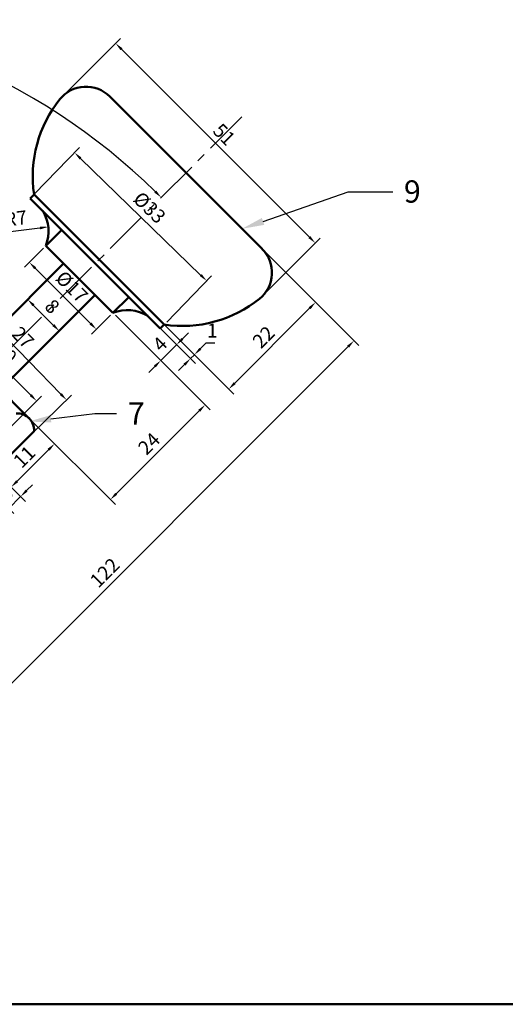
# Model space of a CAD drawing. Units: millimetres. Extents: x -414 to 17, y 81 to 417.
# Tile 5 of 7: x -252 to -165, y 81 to 257. Entities that reach past the tile are written whole.
import ezdxf
from ezdxf import colors
from ezdxf.entities.mleader import LeaderData, LeaderLine
from ezdxf.math import Vec2, Vec3

# ---------------------------------------------------------------- set-up
doc = ezdxf.new("R2010")
doc.units = ezdxf.units.MM
doc.header["$LTSCALE"] = 0.5
doc.linetypes.add('CENTER', pattern=[50.8, 31.75, -6.35, 6.35, -6.35])
for name, color, linetype, lineweight in [('M-CNTR', 1, 'CENTER', 18), ('M-DIMS', 2, 'Continuous', 25), ('M-OUTL', 7, 'Continuous', 50)]:
    doc.layers.add(name, color=color, linetype=linetype, lineweight=lineweight)
doc.styles.get("Standard").update_dxf_attribs({"font": 'arial.ttf'})
doc.dimstyles.new('ISO-25', dxfattribs={"dimtxt": 2.5, "dimasz": 1.5, "dimexe": 1.25, "dimexo": 0.625, "dimtad": 1, "dimtoh": 1, "dimdec": 0, "dimtxsty": 'Standard', "dimcen": 2.5, "dimadec": 0, "dimazin": 0, "dimtfac": 1, "dimtdec": 0, "dimtmove": 0, "dimatfit": 3, "dimfxl": 1, "dimarcsym": 0})

# ---------------------------------------------------------------- blocks, each defined once
blk = doc.blocks.new('*D50')
at = {"layer": 'Defpoints', "color": 0, "ltscale": 0.5, "transparency": 16777216}
for p in [(-244.81, 242.93), (-199.04, 217.13), (-209.03, 207.15)]:
    blk.add_point(p, dxfattribs=at)
at = {"layer": 'M-DIMS', "color": 0, "lineweight": -2, "ltscale": 0.5, "transparency": 16777216}
for p, q in [((-244.37, 243.37), (-233.94, 253.79)), ((-233.77, 251.85), (-200.1, 218.19)), ((-208.58, 207.59), (-198.16, 218.01))]:
    blk.add_line(p, q, dxfattribs=at)
at = {"layer": 'M-DIMS', "color": 0, "ltscale": 0.5, "transparency": 16777216}
for points in [[(-233.59, 252.03), (-233.94, 251.67), (-234.83, 252.91)], [(-199.93, 218.36), (-200.28, 218.01), (-199.04, 217.13)]]:
    blk.add_solid(points, dxfattribs=at)
at = {"layer": 'M-DIMS', "color": 0, "ltscale": 0.5, "transparency": 16777216, "insert": (-215.59, 236.36), "char_height": 2.5, "attachment_point": 5, "rotation": 315}
blk.add_mtext('51', dxfattribs=at)
blk = doc.blocks.new('*D51')
at = {"layer": 'Defpoints', "color": 0, "ltscale": 0.5, "transparency": 16777216}
for p in [(-249.8, 225.49), (-218.51, 210.34), (-226.11, 202.5)]:
    blk.add_point(p, dxfattribs=at)
at = {"layer": 'M-DIMS', "color": 0, "lineweight": -2, "ltscale": 0.5, "transparency": 16777216}
for p, q in [((-249.37, 225.93), (-241.33, 234.22)), ((-241.12, 232.28), (-219.59, 211.39)), ((-225.68, 202.95), (-217.64, 211.24))]:
    blk.add_line(p, q, dxfattribs=at)
at = {"layer": 'M-DIMS', "color": 0, "ltscale": 0.5, "transparency": 16777216}
for points in [[(-240.95, 232.46), (-241.29, 232.1), (-242.2, 233.33)], [(-219.41, 211.57), (-219.76, 211.21), (-218.51, 210.34)]]:
    blk.add_solid(points, dxfattribs=at)
at = {"layer": 'M-DIMS', "color": 0, "ltscale": 0.5, "transparency": 16777216, "insert": (-228.98, 223.25), "char_height": 2.5, "attachment_point": 5, "rotation": 315.8681}
blk.add_mtext('%%C33', dxfattribs=at)
blk = doc.blocks.new('*D52')
at = {"layer": 'Defpoints', "color": 0, "ltscale": 0.5, "transparency": 16777216}
for p in [(-247.33, 216.65), (-235.31, 204.63), (-238.29, 201.65)]:
    blk.add_point(p, dxfattribs=at)
at = {"layer": 'M-DIMS', "color": 0, "lineweight": -2, "ltscale": 0.5, "transparency": 16777216}
for p, q in [((-247.77, 216.2), (-251.19, 212.78)), ((-249.25, 212.61), (-239.35, 202.71)), ((-235.75, 204.18), (-239.17, 200.76))]:
    blk.add_line(p, q, dxfattribs=at)
at = {"layer": 'M-DIMS', "color": 0, "ltscale": 0.5, "transparency": 16777216}
for points in [[(-249.07, 212.78), (-249.42, 212.43), (-250.31, 213.67)], [(-239.17, 202.89), (-239.52, 202.53), (-238.29, 201.65)]]:
    blk.add_solid(points, dxfattribs=at)
at = {"layer": 'M-DIMS', "color": 0, "ltscale": 0.5, "transparency": 16777216, "insert": (-242.9, 209.05), "char_height": 2.5, "attachment_point": 5, "rotation": 315}
blk.add_mtext('%%C17', dxfattribs=at)
blk = doc.blocks.new('*D53')
at = {"layer": 'Defpoints', "color": 0, "ltscale": 0.5, "transparency": 16777216}
for p in [(-250.07, 207.54), (-244.94, 201.36), (-244.41, 201.88)]:
    blk.add_point(p, dxfattribs=at)
at = {"layer": 'M-DIMS', "color": 0, "lineweight": -2, "ltscale": 0.5, "transparency": 16777216}
for p, q in [((-250.51, 207.1), (-251.48, 206.13)), ((-249.54, 205.95), (-246, 202.42)), ((-244.86, 201.44), (-245.82, 200.47))]:
    blk.add_line(p, q, dxfattribs=at)
at = {"layer": 'M-DIMS', "color": 0, "ltscale": 0.5, "transparency": 16777216}
for points in [[(-249.36, 206.13), (-249.71, 205.78), (-250.6, 207.01)], [(-245.82, 202.59), (-246.18, 202.24), (-244.94, 201.36)]]:
    blk.add_solid(points, dxfattribs=at)
at = {"layer": 'M-DIMS', "color": 0, "ltscale": 0.5, "transparency": 16777216, "insert": (-246.42, 205.53), "char_height": 2.5, "attachment_point": 5, "rotation": 315}
blk.add_mtext('8', dxfattribs=at)
blk = doc.blocks.new('*D54')
at = {"layer": 'Defpoints', "color": 0, "ltscale": 0.5, "transparency": 16777216}
for p in [(-212.18, 219.68), (-199, 206.5), (-227.73, 204.12)]:
    blk.add_point(p, dxfattribs=at)
at = {"layer": 'M-DIMS', "color": 0, "lineweight": -2, "ltscale": 0.5, "transparency": 16777216}
for p, q in [((-211.74, 219.24), (-198.11, 205.62)), ((-213.49, 192), (-200.06, 205.44)), ((-227.29, 203.68), (-213.67, 190.06))]:
    blk.add_line(p, q, dxfattribs=at)
at = {"layer": 'M-DIMS', "color": 0, "ltscale": 0.5, "transparency": 16777216}
for points in [[(-200.23, 205.62), (-199.88, 205.26), (-199, 206.5)], [(-213.67, 192.18), (-213.32, 191.83), (-214.55, 190.94)]]:
    blk.add_solid(points, dxfattribs=at)
at = {"layer": 'M-DIMS', "color": 0, "ltscale": 0.5, "transparency": 16777216, "insert": (-208.1, 200.05), "char_height": 2.5, "attachment_point": 5, "rotation": 45}
blk.add_mtext('22', dxfattribs=at)
blk = doc.blocks.new('*D55')
at = {"layer": 'Defpoints', "color": 0, "ltscale": 0.5, "transparency": 16777216}
for p in [(-226.82, 201.8), (-226.11, 202.5), (-221.42, 196.4)]:
    blk.add_point(p, dxfattribs=at)
at = {"layer": 'M-DIMS', "color": 0, "lineweight": -2, "ltscale": 0.5, "transparency": 16777216}
for p, q in [((-226.38, 201.36), (-220.54, 195.51)), ((-225.67, 202.06), (-219.83, 196.22)), ((-219.65, 198.16), (-218.59, 199.22)), ((-218.59, 199.22), (-217.05, 199.22)), ((-221.42, 196.4), (-220.71, 197.1)), ((-222.48, 195.34), (-223.54, 194.27))]:
    blk.add_line(p, q, dxfattribs=at)
at = {"layer": 'M-DIMS', "color": 0, "ltscale": 0.5, "transparency": 16777216}
for points in [[(-219.83, 198.34), (-219.48, 197.99), (-220.71, 197.1)], [(-222.66, 195.51), (-222.3, 195.16), (-221.42, 196.4)]]:
    blk.add_solid(points, dxfattribs=at)
at = {"layer": 'M-DIMS', "color": 0, "ltscale": 0.5, "transparency": 16777216, "insert": (-217.51, 201.1), "char_height": 2.5, "attachment_point": 5}
blk.add_mtext('1', dxfattribs=at)
blk = doc.blocks.new('*D56')
at = {"layer": 'Defpoints', "color": 0, "ltscale": 0.5, "transparency": 16777216}
for p in [(-232.48, 207.45), (-235.31, 204.63), (-223.92, 198.89)]:
    blk.add_point(p, dxfattribs=at)
at = {"layer": 'M-DIMS', "color": 0, "lineweight": -2, "ltscale": 0.5, "transparency": 16777216}
for p, q in [((-232.04, 207.01), (-223.03, 198.01)), ((-234.87, 204.18), (-225.86, 195.18)), ((-222.86, 199.95), (-221.8, 201.01)), ((-226.75, 196.06), (-223.92, 198.89)), ((-227.81, 195), (-228.87, 193.94))]:
    blk.add_line(p, q, dxfattribs=at)
at = {"layer": 'M-DIMS', "color": 0, "ltscale": 0.5, "transparency": 16777216}
for points in [[(-223.03, 200.13), (-222.68, 199.78), (-223.92, 198.89)], [(-227.98, 195.18), (-227.63, 194.83), (-226.75, 196.06)]]:
    blk.add_solid(points, dxfattribs=at)
at = {"layer": 'M-DIMS', "color": 0, "ltscale": 0.5, "transparency": 16777216, "insert": (-226.66, 198.8), "char_height": 2.5, "attachment_point": 5, "rotation": 45}
blk.add_mtext('4', dxfattribs=at)
blk = doc.blocks.new('*D57')
at = {"layer": 'Defpoints', "color": 0, "ltscale": 0.5, "transparency": 16777216}
for p in [(-253.85, 219.19), (-246.9, 220.01)]:
    blk.add_point(p, dxfattribs=at)
at = {"layer": 'M-DIMS', "color": 0, "lineweight": -2, "ltscale": 0.5, "transparency": 16777216}
blk.add_line((-255.12, 219.04), (-248.39, 219.83), dxfattribs=at)
at = {"layer": 'M-DIMS', "color": 0, "ltscale": 0.5, "transparency": 16777216}
blk.add_solid([(-248.42, 220.08), (-248.36, 219.58), (-246.9, 220.01)], dxfattribs=at)
at = {"layer": 'M-DIMS', "color": 0, "ltscale": 0.5, "transparency": 16777216, "insert": (-252.72, 221.21), "char_height": 2.5, "attachment_point": 5, "rotation": 6.7279}
blk.add_mtext('R7', dxfattribs=at)
blk = doc.blocks.new('*D58')
at = {"layer": 'Defpoints', "color": 0, "ltscale": 0.5, "transparency": 16777216}
for p in [(-233.2, 202.52), (-218.79, 188.11), (-250.18, 185.54)]:
    blk.add_point(p, dxfattribs=at)
at = {"layer": 'M-DIMS', "color": 0, "lineweight": -2, "ltscale": 0.5, "transparency": 16777216}
for p, q in [((-232.76, 202.08), (-217.91, 187.23)), ((-234.71, 172.19), (-219.85, 187.05)), ((-249.73, 185.1), (-234.88, 170.25))]:
    blk.add_line(p, q, dxfattribs=at)
at = {"layer": 'M-DIMS', "color": 0, "ltscale": 0.5, "transparency": 16777216}
for points in [[(-220.03, 187.23), (-219.67, 186.87), (-218.79, 188.11)], [(-234.88, 172.37), (-234.53, 172.02), (-235.77, 171.13)]]:
    blk.add_solid(points, dxfattribs=at)
at = {"layer": 'M-DIMS', "color": 0, "ltscale": 0.5, "transparency": 16777216, "insert": (-228.61, 180.95), "char_height": 2.5, "attachment_point": 5, "rotation": 45}
blk.add_mtext('24', dxfattribs=at)
blk = doc.blocks.new('*D59')
at = {"layer": 'Defpoints', "color": 0, "ltscale": 0.5, "transparency": 16777216}
for p in [(-250.18, 185.54), (-257.95, 177.77), (-253.55, 173.37)]:
    blk.add_point(p, dxfattribs=at)
at = {"layer": 'M-DIMS', "color": 0, "lineweight": -2, "ltscale": 0.5, "transparency": 16777216}
for p, q in [((-249.73, 185.1), (-244.89, 180.26)), ((-246.84, 180.08), (-252.49, 174.43)), ((-257.51, 177.33), (-252.67, 172.49))]:
    blk.add_line(p, q, dxfattribs=at)
at = {"layer": 'M-DIMS', "color": 0, "ltscale": 0.5, "transparency": 16777216}
for points in [[(-247.02, 180.26), (-246.66, 179.91), (-245.78, 181.14)], [(-252.67, 174.61), (-252.31, 174.26), (-253.55, 173.37)]]:
    blk.add_solid(points, dxfattribs=at)
at = {"layer": 'M-DIMS', "color": 0, "ltscale": 0.5, "transparency": 16777216, "insert": (-250.99, 178.59), "char_height": 2.5, "attachment_point": 5, "rotation": 45}
blk.add_mtext('11', dxfattribs=at)
blk = doc.blocks.new('*D60')
at = {"layer": 'Defpoints', "color": 0, "ltscale": 0.5, "transparency": 16777216}
for p in [(-271.72, 199.32), (-243.63, 188.99), (-252.89, 179.97)]:
    blk.add_point(p, dxfattribs=at)
at = {"layer": 'M-DIMS', "color": 0, "lineweight": -2, "ltscale": 0.5, "transparency": 16777216}
for p, q in [((-271.28, 199.76), (-261.56, 209.21)), ((-261.41, 207.26), (-244.67, 190.06)), ((-252.45, 180.4), (-242.73, 189.86))]:
    blk.add_line(p, q, dxfattribs=at)
at = {"layer": 'M-DIMS', "color": 0, "ltscale": 0.5, "transparency": 16777216}
for points in [[(-261.23, 207.44), (-261.59, 207.09), (-262.46, 208.34)], [(-244.49, 190.23), (-244.85, 189.89), (-243.63, 188.99)]]:
    blk.add_solid(points, dxfattribs=at)
at = {"layer": 'M-DIMS', "color": 0, "ltscale": 0.5, "transparency": 16777216, "insert": (-251.69, 199.97), "char_height": 2.5, "attachment_point": 5, "rotation": 314.2138}
blk.add_mtext('27', dxfattribs=at)
blk = doc.blocks.new('*D61')
at = {"layer": 'Defpoints', "color": 0, "ltscale": 0.5, "transparency": 16777216}
for p in [(-274.2, 191.9), (-249, 188.81), (-260.06, 177.76)]:
    blk.add_point(p, dxfattribs=at)
at = {"layer": 'M-DIMS', "color": 0, "lineweight": -2, "ltscale": 0.5, "transparency": 16777216}
for p, q in [((-273.76, 192.34), (-262.26, 203.84)), ((-262.08, 201.89), (-250.06, 189.87)), ((-259.61, 178.2), (-248.12, 189.7))]:
    blk.add_line(p, q, dxfattribs=at)
at = {"layer": 'M-DIMS', "color": 0, "ltscale": 0.5, "transparency": 16777216}
for points in [[(-261.9, 202.07), (-262.26, 201.72), (-263.14, 202.95)], [(-249.88, 190.05), (-250.24, 189.7), (-249, 188.81)]]:
    blk.add_solid(points, dxfattribs=at)
at = {"layer": 'M-DIMS', "color": 0, "ltscale": 0.5, "transparency": 16777216, "insert": (-254.73, 197.23), "char_height": 2.5, "attachment_point": 5, "rotation": 315}
blk.add_mtext('20', dxfattribs=at)
blk = doc.blocks.new('*D67')
at = {"layer": 'Defpoints', "color": 0, "ltscale": 0.5, "transparency": 16777216}
for p in [(-259, 178.82), (-261.12, 176.7), (-251.86, 171.68)]:
    blk.add_point(p, dxfattribs=at)
at = {"layer": 'M-DIMS', "color": 0, "lineweight": -2, "ltscale": 0.5, "transparency": 16777216}
for p, q in [((-258.55, 178.37), (-250.97, 170.8)), ((-260.67, 176.25), (-253.1, 168.67)), ((-250.8, 172.74), (-249.74, 173.8)), ((-253.98, 169.56), (-251.86, 171.68)), ((-255.04, 168.5), (-256.1, 167.44))]:
    blk.add_line(p, q, dxfattribs=at)
at = {"layer": 'M-DIMS', "color": 0, "ltscale": 0.5, "transparency": 16777216}
for points in [[(-250.97, 172.92), (-250.62, 172.56), (-251.86, 171.68)], [(-255.22, 168.67), (-254.86, 168.32), (-253.98, 169.56)]]:
    blk.add_solid(points, dxfattribs=at)
at = {"layer": 'M-DIMS', "color": 0, "ltscale": 0.5, "transparency": 16777216, "insert": (-254.26, 171.96), "char_height": 2.5, "attachment_point": 5, "rotation": 45}
blk.add_mtext('3', dxfattribs=at)
blk = doc.blocks.new('*D70')
at = {"layer": 'Defpoints', "color": 0, "ltscale": 0.5, "transparency": 16777216}
for p in [(-222.23, 229.73), (-308.49, 143.46), (-278.37, 113.34)]:
    blk.add_point(p, dxfattribs=at)
at = {"layer": 'M-DIMS', "color": 0, "lineweight": -2, "ltscale": 0.5, "transparency": 16777216}
for p, q in [((-221.78, 229.29), (-191.22, 198.73)), ((-193.17, 198.55), (-277.31, 114.4)), ((-308.05, 143.02), (-277.49, 112.46))]:
    blk.add_line(p, q, dxfattribs=at)
at = {"layer": 'M-DIMS', "color": 0, "ltscale": 0.5, "transparency": 16777216}
for points in [[(-193.34, 198.73), (-192.99, 198.37), (-192.11, 199.61)], [(-277.49, 114.58), (-277.14, 114.23), (-278.37, 113.34)]]:
    blk.add_solid(points, dxfattribs=at)
at = {"layer": 'M-DIMS', "color": 0, "ltscale": 0.5, "transparency": 16777216, "insert": (-236.57, 157.81), "char_height": 2.5, "attachment_point": 5, "rotation": 45}
blk.add_mtext('122', dxfattribs=at)
blk = doc.blocks.new('*D78')
at = {"layer": 'Defpoints', "color": 0, "ltscale": 0.5, "transparency": 16777216}
for p in [(-308.49, 365.43), (-250.63, 243.68), (-212.22, 239.73), (-308.49, 230.96), (-308.49, 143.46)]:
    blk.add_point(p, dxfattribs=at)
at = {"layer": 'M-DIMS', "color": 0, "lineweight": -2, "ltscale": 0.5, "transparency": 16777216}
blk.add_arc((-308.49, 143.46), 115.73, 45.7426, 89.2574, dxfattribs=at)
at = {"layer": 'M-DIMS', "color": 0, "ltscale": 0.5, "transparency": 16777216}
for points in [[(-306.99, 258.93), (-306.99, 259.43), (-308.49, 259.19)], [(-227.55, 226.52), (-227.9, 226.17), (-226.66, 225.29)]]:
    blk.add_solid(points, dxfattribs=at)
at = {"layer": 'M-DIMS', "color": 0, "ltscale": 0.5, "transparency": 16777216, "insert": (-263.48, 252.13), "char_height": 2.5, "attachment_point": 5, "rotation": 337.5}
blk.add_mtext('45°', dxfattribs=at)

msp = doc.modelspace()

# ---------------------------------------------------------------- linework, layer by layer
at = {"layer": 'M-CNTR', "ltscale": 0.5}
msp.add_line((-212.22, 239.73), (-308.49, 143.46), dxfattribs=at)
at = {"layer": 'M-OUTL', "ltscale": 0.5}
for p, q in [((-235.9, 243.4), (-208.55, 216.06)), ((-250.16, 225.13), (-249.45, 225.84)), ((-250.16, 225.13), (-226.82, 201.8)), ((-250.16, 225.13), (-226.82, 201.8)), ((-249.45, 225.84), (-226.11, 202.5)), ((-247.33, 216.65), (-244.5, 219.48)), ((-247.33, 216.65), (-235.31, 204.63)), ((-261.12, 196.49), (-244.15, 213.46)), ((-238.49, 207.81), (-255.46, 190.84)), ((-232.48, 207.45), (-235.31, 204.63)), ((-266.3, 201.68), (-250.32, 185.7)), ((-226.11, 202.5), (-226.82, 201.8)), ((-249.45, 183.41), (-255.81, 177.05))]:
    msp.add_line(p, q, dxfattribs=at)
msp.add_lwpolyline([(-414.36, 417.09), (16.87, 417.09), (16.87, 80.66), (-414.36, 80.66)], close=True, dxfattribs=at)
for centre, radius, start, end in [((-240.14, 239.16), 6, 45, 141.0758), ((-227.69, 229.11), 22, 141.0758, 188.5379), ((-253.85, 219.19), 7, 338.7269, 31.857), ((-212.8, 211.81), 6, 308.9242, 45), ((-222.85, 224.26), 22, 261.4621, 308.9242), ((-232.77, 198.1), 7, 58.143, 111.2731), ((-252.48, 183.57), 3.03, 357.0731, 92.9269)]:
    msp.add_arc(centre, radius, start, end, dxfattribs=at)

# ---------------------------------------------------------------- dimensions: what is measured, and where the dimension line sits
at = {"layer": 'M-DIMS', "ltscale": 0.5}
dim = msp.add_angular_dim_2l(base=(-250.63, 243.68), line1=((-308.49, 365.43), (-308.49, 230.96)), line2=((-212.22, 239.73), (-308.49, 143.46)), dimstyle='ISO-25', override={"dimclrd": 0, "dimclre": 0, "dimclrt": 0}, dxfattribs=at)
dim.commit()
dim.dimension.update_dxf_attribs({"geometry": '*D78', "text_midpoint": (-263.48, 252.13)})
for p1, p2, distance, picture, middle in [((-244.81, 242.93), (-209.03, 207.15), 14.12, '*D50', (-215.59, 236.36)), ((-222.23, 229.73), (-308.49, 143.46), 42.59, '*D70', (-236.57, 157.81)), ((-227.73, 204.12), (-212.18, 219.68), -18.64, '*D54', (-208.1, 200.05)), ((-271.72, 199.32), (-252.89, 179.97), 12.93, '*D60', (-251.69, 199.97)), ((-250.07, 207.54), (-244.41, 201.88), -0.75, '*D53', (-246.42, 205.53)), ((-235.31, 204.63), (-232.48, 207.45), -12.11, '*D56', (-226.66, 198.8)), ((-274.2, 191.9), (-260.06, 177.76), 15.64, '*D61', (-254.73, 197.23)), ((-250.18, 185.54), (-233.2, 202.52), -20.38, '*D58', (-228.61, 180.95)), ((-250.18, 185.54), (-257.95, 177.77), 6.22, '*D59', (-250.99, 178.59)), ((-261.12, 176.7), (-259, 178.82), -10.09, '*D67', (-254.26, 171.96))]:
    dim = msp.add_aligned_dim(p1=p1, p2=p2, distance=distance, dimstyle='ISO-25', override={"dimclrd": 0, "dimclre": 0, "dimclrt": 0}, dxfattribs=at)
    dim.commit()
    dim.dimension.update_dxf_attribs({"geometry": picture, "text_midpoint": middle})
for p1, p2, distance, picture, middle in [((-249.8, 225.49), (-226.11, 202.5), 10.92, '*D51', (-228.98, 223.25)), ((-247.33, 216.65), (-235.31, 204.63), -4.21, '*D52', (-242.9, 209.05))]:
    dim = msp.add_aligned_dim(p1=p1, p2=p2, distance=distance, text='%%C<>', dimstyle='ISO-25', override={"dimclrd": 0, "dimclre": 0, "dimclrt": 0}, dxfattribs=at)
    dim.commit()
    dim.dimension.update_dxf_attribs({"geometry": picture, "text_midpoint": middle})
dim = msp.add_radius_dim(center=(-253.85, 219.19), mpoint=(-246.9, 220.01), dimstyle='ISO-25', override={"dimclrd": 0, "dimclre": 0, "dimclrt": 0}, dxfattribs=at)
dim.commit()
dim.dimension.update_dxf_attribs({"geometry": '*D57', "text_midpoint": (-252.5, 219.35), "dimtype": 164})
dim = msp.add_linear_dim(base=(-221.42, 196.4), p1=(-226.11, 202.5), p2=(-226.82, 201.8), angle=225, dimstyle='ISO-25', override={"dimclrd": 0, "dimclre": 0, "dimclrt": 0}, dxfattribs=at)
dim.commit()
dim.dimension.update_dxf_attribs({"geometry": '*D55', "text_midpoint": (-217.51, 199.22), "dimtype": 161})

# ---------------------------------------------------------------- leaders
ml = msp.add_multileader_mtext('Standard', dxfattribs=at)
ml.set_content('9', color=256)
ml.set_leader_properties()
ml.build(insert=Vec2(0, 0))
ctx = ml.context
ctx.base_point, ctx.plane_origin = Vec3(-185.16, 226.33), Vec3(-212.18, 219.68)
notes = []
notes.append((ctx, [(0, (1, 1, 0), (-193.16, 226.33), (1, 0), 8, [(0, [(-212.18, 219.68)], 0, [])])]))
ctx.mtext.insert, ctx.mtext.flow_direction = Vec3(-183.16, 228.36), 5
ml = msp.add_multileader_mtext('Standard', dxfattribs=at)
ml.set_content('7', color=256)
ml.set_leader_properties()
ml.build(insert=Vec2(0, 0))
ctx = ml.context
ctx.base_point, ctx.plane_origin = Vec3(-234.65, 186.55), Vec3(-250.41, 185.13)
notes.append((ctx, [(0, (1, 1, 0), (-238.56, 186.55), (1, 0), 3.91, [(0, [(-250.41, 185.13)], 0, [])])]))
ctx.mtext.insert, ctx.mtext.flow_direction = Vec3(-232.65, 188.55), 5
for ctx, leaders in notes:
    for number, flags, end, landing, length, lines in leaders:
        leader = LeaderData()
        leader.index, (leader.has_last_leader_line, leader.has_dogleg_vector, leader.attachment_direction) = number, flags
        leader.last_leader_point, leader.dogleg_vector, leader.dogleg_length = Vec3(end), Vec3(landing), length
        for number, points, colour, breaks in lines:
            line = LeaderLine()
            line.index, line.vertices, line.color, line.breaks = number, Vec3.list(points), colors.encode_raw_color(colour), breaks
            leader.lines.append(line)
        ctx.leaders.append(leader)

doc.saveas('drawing.dxf')
